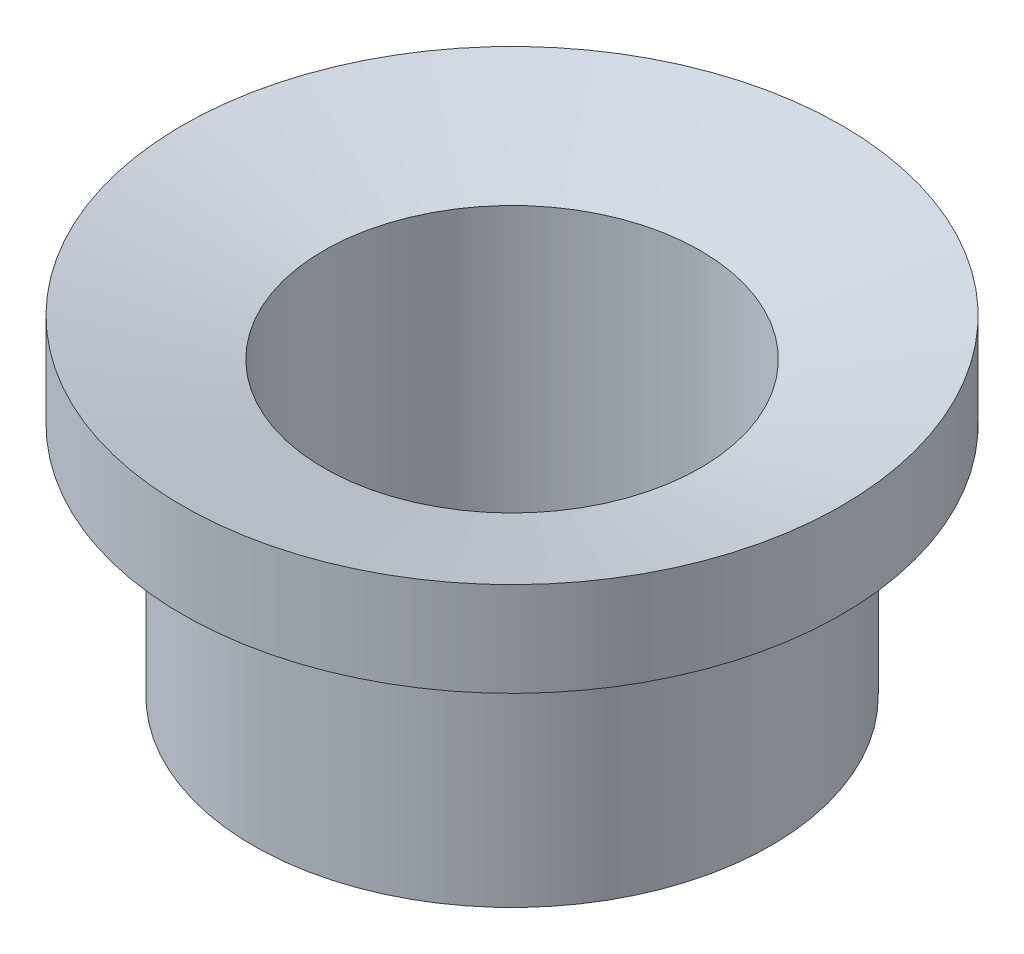
ISO-10303-21;
HEADER;
FILE_DESCRIPTION(('STEP AP214'),'2;1');
FILE_NAME('part.step','',(''),(''),'','','');
FILE_SCHEMA(('AUTOMOTIVE_DESIGN { 1 0 10303 214 1 1 1 1 }'));
ENDSEC;
DATA;
#1=APPLICATION_CONTEXT('core data for automotive mechanical design processes');
#2=APPLICATION_PROTOCOL_DEFINITION('international standard','automotive_design',2000,#1);
#3=PRODUCT_CONTEXT('',#1,'mechanical');
#4=PRODUCT('Part','Part','',(#3));
#5=PRODUCT_RELATED_PRODUCT_CATEGORY('part','',(#4));
#6=PRODUCT_DEFINITION_FORMATION('','',#4);
#7=PRODUCT_DEFINITION_CONTEXT('part definition',#1,'design');
#8=PRODUCT_DEFINITION('design','',#6,#7);
#9=PRODUCT_DEFINITION_SHAPE('','',#8);
#10=(LENGTH_UNIT() NAMED_UNIT(*) SI_UNIT(.MILLI.,.METRE.));
#11=(NAMED_UNIT(*) PLANE_ANGLE_UNIT() SI_UNIT($,.RADIAN.));
#12=(NAMED_UNIT(*) SI_UNIT($,.STERADIAN.) SOLID_ANGLE_UNIT());
#13=UNCERTAINTY_MEASURE_WITH_UNIT(LENGTH_MEASURE(1.E-05),#10,'distance_accuracy_value','');
#14=(GEOMETRIC_REPRESENTATION_CONTEXT(3) GLOBAL_UNCERTAINTY_ASSIGNED_CONTEXT((#13)) GLOBAL_UNIT_ASSIGNED_CONTEXT((#10,
#11,#12)) REPRESENTATION_CONTEXT('',''));
#15=CARTESIAN_POINT('',(0.,0.,0.));
#16=DIRECTION('',(0.,0.,1.));
#17=DIRECTION('',(1.,0.,0.));
#18=AXIS2_PLACEMENT_3D('',#15,#16,#17);
#19=CARTESIAN_POINT('',(-16.5,0.,0.));
#20=DIRECTION('',(0.,1.,0.));
#21=DIRECTION('',(0.,0.,1.));
#22=AXIS2_PLACEMENT_3D('',#19,#20,#21);
#23=PLANE('',#22);
#24=CARTESIAN_POINT('',(0.,0.,0.));
#25=DIRECTION('',(0.,-1.,0.));
#26=DIRECTION('',(0.,0.,-1.));
#27=AXIS2_PLACEMENT_3D('',#24,#25,#26);
#28=CIRCLE('',#27,12.);
#29=CARTESIAN_POINT('',(0.,0.,-12.));
#30=VERTEX_POINT('',#29);
#31=EDGE_CURVE('E10',#30,#30,#28,.T.);
#32=ORIENTED_EDGE('',*,*,#31,.F.);
#33=EDGE_LOOP('',(#32));
#34=FACE_BOUND('',#33,.T.);
#35=CARTESIAN_POINT('',(0.,0.,0.));
#36=DIRECTION('',(0.,-1.,0.));
#37=DIRECTION('',(0.,0.,-1.));
#38=AXIS2_PLACEMENT_3D('',#35,#36,#37);
#39=CIRCLE('',#38,16.5);
#40=CARTESIAN_POINT('',(0.,0.,-16.5));
#41=VERTEX_POINT('',#40);
#42=EDGE_CURVE('E56',#41,#41,#39,.T.);
#43=ORIENTED_EDGE('',*,*,#42,.T.);
#44=EDGE_LOOP('',(#43));
#45=FACE_BOUND('',#44,.T.);
#46=ADVANCED_FACE('F40',(#34,#45),#23,.F.);
#47=CARTESIAN_POINT('',(0.,-13.8695652173913,0.));
#48=DIRECTION('',(0.,-1.,0.));
#49=DIRECTION('',(0.,0.,-1.));
#50=AXIS2_PLACEMENT_3D('',#47,#48,#49);
#51=CYLINDRICAL_SURFACE('',#50,12.);
#52=CARTESIAN_POINT('',(0.,18.58845726812,0.));
#53=DIRECTION('',(0.,-1.,0.));
#54=DIRECTION('',(0.,0.,-1.));
#55=AXIS2_PLACEMENT_3D('',#52,#53,#54);
#56=CIRCLE('',#55,12.);
#57=CARTESIAN_POINT('',(0.,18.58845726812,-12.));
#58=VERTEX_POINT('',#57);
#59=EDGE_CURVE('E43',#58,#58,#56,.T.);
#60=ORIENTED_EDGE('',*,*,#59,.F.);
#61=EDGE_LOOP('',(#60));
#62=FACE_BOUND('',#61,.T.);
#63=ORIENTED_EDGE('',*,*,#31,.T.);
#64=EDGE_LOOP('',(#63));
#65=FACE_BOUND('',#64,.T.);
#66=ADVANCED_FACE('F82',(#62,#65),#51,.F.);
#67=CARTESIAN_POINT('',(0.,18.58845726812,0.));
#68=DIRECTION('',(0.,1.,0.));
#69=DIRECTION('',(0.,0.,1.));
#70=AXIS2_PLACEMENT_3D('',#67,#68,#69);
#71=CONICAL_SURFACE('',#70,12.,1.30899693899575);
#72=CARTESIAN_POINT('',(0.,21.,0.));
#73=DIRECTION('',(0.,-1.,0.));
#74=DIRECTION('',(0.,0.,-1.));
#75=AXIS2_PLACEMENT_3D('',#72,#73,#74);
#76=CIRCLE('',#75,21.);
#77=CARTESIAN_POINT('',(0.,21.,-21.));
#78=VERTEX_POINT('',#77);
#79=EDGE_CURVE('E50',#78,#78,#76,.T.);
#80=ORIENTED_EDGE('',*,*,#79,.F.);
#81=EDGE_LOOP('',(#80));
#82=FACE_BOUND('',#81,.T.);
#83=ORIENTED_EDGE('',*,*,#59,.T.);
#84=EDGE_LOOP('',(#83));
#85=FACE_BOUND('',#84,.T.);
#86=ADVANCED_FACE('F76',(#82,#85),#71,.F.);
#87=CARTESIAN_POINT('',(0.,-13.8695652173913,0.));
#88=DIRECTION('',(0.,-1.,0.));
#89=DIRECTION('',(0.,0.,-1.));
#90=AXIS2_PLACEMENT_3D('',#87,#88,#89);
#91=CYLINDRICAL_SURFACE('',#90,21.);
#92=CARTESIAN_POINT('',(0.,15.,0.));
#93=DIRECTION('',(0.,-1.,0.));
#94=DIRECTION('',(0.,0.,-1.));
#95=AXIS2_PLACEMENT_3D('',#92,#93,#94);
#96=CIRCLE('',#95,21.);
#97=CARTESIAN_POINT('',(0.,15.,-21.));
#98=VERTEX_POINT('',#97);
#99=EDGE_CURVE('E51',#98,#98,#96,.T.);
#100=ORIENTED_EDGE('',*,*,#99,.F.);
#101=EDGE_LOOP('',(#100));
#102=FACE_BOUND('',#101,.T.);
#103=ORIENTED_EDGE('',*,*,#79,.T.);
#104=EDGE_LOOP('',(#103));
#105=FACE_BOUND('',#104,.T.);
#106=ADVANCED_FACE('F71',(#102,#105),#91,.T.);
#107=CARTESIAN_POINT('',(-21.,15.,0.));
#108=DIRECTION('',(0.,1.,0.));
#109=DIRECTION('',(0.,0.,1.));
#110=AXIS2_PLACEMENT_3D('',#107,#108,#109);
#111=PLANE('',#110);
#112=CARTESIAN_POINT('',(0.,15.,0.));
#113=DIRECTION('',(0.,-1.,0.));
#114=DIRECTION('',(0.,0.,-1.));
#115=AXIS2_PLACEMENT_3D('',#112,#113,#114);
#116=CIRCLE('',#115,16.5);
#117=CARTESIAN_POINT('',(0.,15.,-16.5));
#118=VERTEX_POINT('',#117);
#119=EDGE_CURVE('E57',#118,#118,#116,.T.);
#120=ORIENTED_EDGE('',*,*,#119,.F.);
#121=EDGE_LOOP('',(#120));
#122=FACE_BOUND('',#121,.T.);
#123=ORIENTED_EDGE('',*,*,#99,.T.);
#124=EDGE_LOOP('',(#123));
#125=FACE_BOUND('',#124,.T.);
#126=ADVANCED_FACE('F70',(#122,#125),#111,.F.);
#127=CARTESIAN_POINT('',(0.,-13.8695652173913,0.));
#128=DIRECTION('',(0.,-1.,0.));
#129=DIRECTION('',(0.,0.,-1.));
#130=AXIS2_PLACEMENT_3D('',#127,#128,#129);
#131=CYLINDRICAL_SURFACE('',#130,16.5);
#132=ORIENTED_EDGE('',*,*,#42,.F.);
#133=EDGE_LOOP('',(#132));
#134=FACE_BOUND('',#133,.T.);
#135=ORIENTED_EDGE('',*,*,#119,.T.);
#136=EDGE_LOOP('',(#135));
#137=FACE_BOUND('',#136,.T.);
#138=ADVANCED_FACE('F61',(#134,#137),#131,.T.);
#139=CLOSED_SHELL('',(#46,#66,#86,#106,#126,#138));
#140=MANIFOLD_SOLID_BREP('B2',#139);
#141=ADVANCED_BREP_SHAPE_REPRESENTATION('',(#18,#140),#14);
#142=SHAPE_DEFINITION_REPRESENTATION(#9,#141);
ENDSEC;
END-ISO-10303-21;
